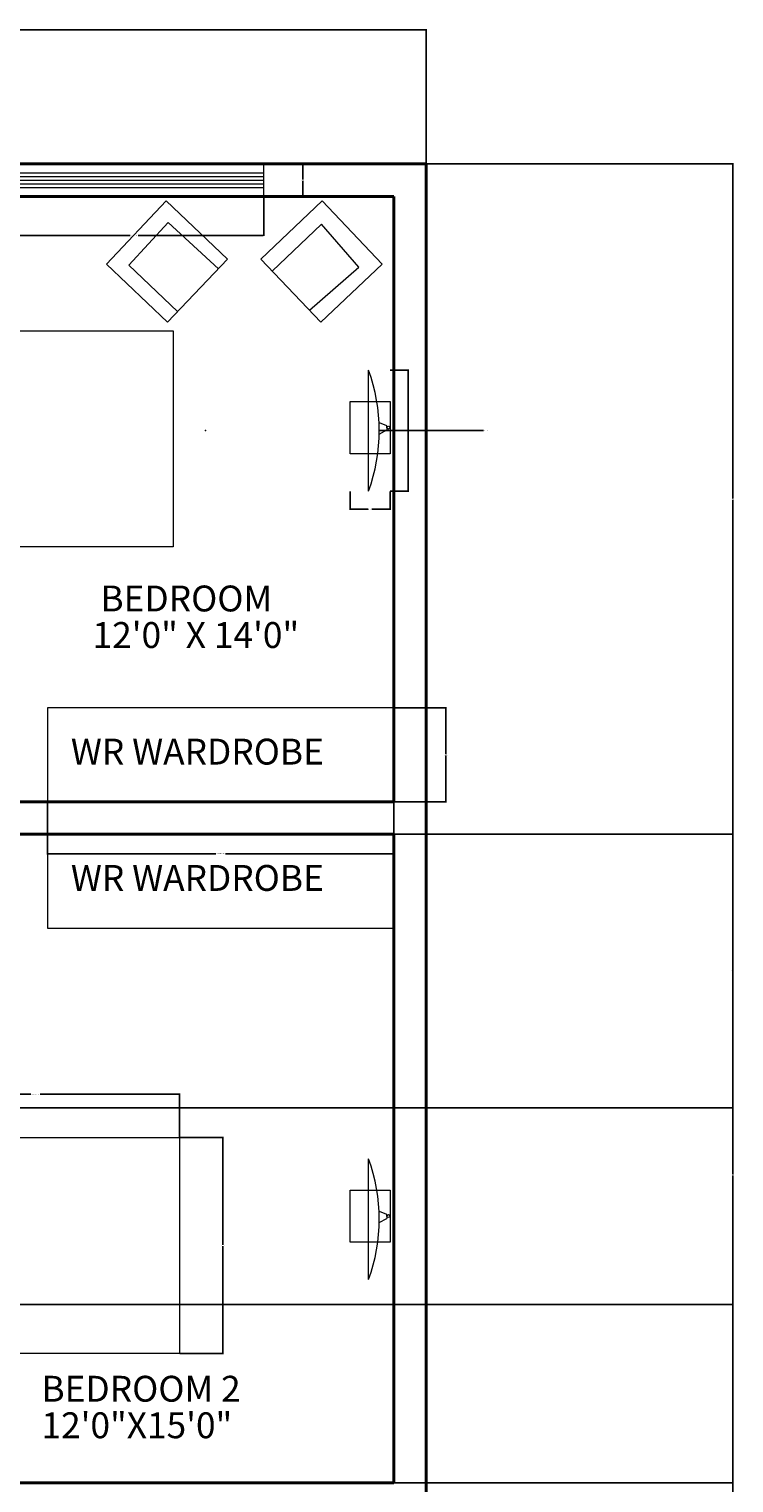
# Model space of a CAD drawing. Units: inches. Extents: x 12978 to 13669, y 46550 to 47327.
# Tile 5 of 5: x 13474 to 13669, y 46901 to 47304. Entities that reach past the tile are written whole.
import ezdxf

# ---------------------------------------------------------------- set-up
doc = ezdxf.new("R2010")
doc.units = ezdxf.units.IN
for name, color, linetype, lineweight in [('A-ANNO-DIMS', 2, 'Continuous', 18), ('A-AREA-IDEN', 1, 'Continuous', 18), ('A-EQPM', 8, 'Continuous', 18), ('A-FLOR-CASE', 8, 'Continuous', 20), ('furniture', 5, 'Continuous', 18), ('text', 1, 'Continuous', 18), ('wall', 7, 'Continuous', 40), ('window', 1, 'Continuous', 18)]:
    doc.layers.add(name, color=color, linetype=linetype, lineweight=lineweight)
doc.styles.get("Standard").update_dxf_attribs({"font": 'arial.ttf'})
doc.dimstyles.get("Standard").update_dxf_attribs({"dimtxt": 0.18, "dimasz": 0.18, "dimexe": 0.18, "dimexo": 0.0625, "dimgap": 0.09, "dimtad": 0, "dimtih": 1, "dimtoh": 1, "dimdec": 4, "dimzin": 0, "dimdsep": 46, "dimtxsty": 'Standard', "dimcen": 0.09, "dimadec": 0, "dimazin": 0, "dimtfac": 1, "dimtdec": 4, "dimtofl": 0, "dimtmove": 0, "dimatfit": 3, "dimfxl": 1, "dimtolj": 1, "dimtzin": 0, "dimarcsym": 0})

# ---------------------------------------------------------------- blocks, each defined once
blk = doc.blocks.new('Bed - Queen')
for p, q in [((0, -80.00003), (0, 0)), ((0, 0), (59.99999, 0)), ((59.99999, 0), (59.99999, -80.00003)), ((7.99999, -1.2), (28.79998, -1.2)), ((7.99999, -14.4), (7.99999, -1.2)), ((28.79998, -1.2), (28.79998, -14.4)), ((31.19999, -1.2), (51.99999, -1.2)), ((31.19999, -14.4), (31.19999, -1.2)), ((51.99999, -1.2), (51.99999, -16.4)), ((0, -14.4), (44.8, -14.4)), ((59.99999, -29.6), (44.8, -14.4)), ((44.8, -14.4), (44.8, -29.6)), ((44.8, -16.8), (0, -16.8)), ((51.99999, -16.4), (46.79936, -16.4)), ((44.8, -29.6), (59.99999, -29.6)), ((59.99999, -80.00003), (0, -80.00003))]:
    blk.add_line(p, q)
blk = doc.blocks.new('WINDOW-72')
for p, q in [((0, 0), (0, 9)), ((72, 0), (72, 9)), ((0, 6.5), (72, 6.5)), ((0, 5.5), (72, 5.5)), ((0, 4.5), (72, 4.5)), ((0, 3.5), (72, 3.5)), ((0, 2.5), (72, 2.5))]:
    blk.add_line(p, q)
blk = doc.blocks.new('TV-FLATSCREEN')
for p, q in [((5.09, 0), (5.09, 33.56)), ((8.05, 19.02), (10.09, 18.18)), ((8.09, 15.82), (10.22, 17.01)), ((10.09, 18.18), (10.22, 17.01)), ((11.07, 17.34), (11.07, 18.07))]:
    blk.add_line(p, q)
blk.add_lwpolyline([(0, 24.86), (11.07, 24.86), (11.07, 10.37), (0, 10.37)], close=True)
blk.add_circle((10.63, 17.63), 0.418)
blk.add_arc((-40.12, 16.78), 48.22, 339.6348, 20.3652)
blk = doc.blocks.new('WARDROBE-96')
blk.add_lwpolyline([(0, 0), (96.12, 0), (96.12, 26.05), (0, 26.05)], close=True)
blk = doc.blocks.new('*D23')
at = {"layer": 'A-ANNO-DIMS', "color": 0, "lineweight": -2, "transparency": 16777216}
for p, q in [((13435.54, 46996.57), (13435.54, 47008.69)), ((13435.72, 47008.51), (13474.24, 47008.51)), ((13515.36, 47008.51), (13476.84, 47008.51)), ((13515.54, 46996.57), (13515.54, 47008.69))]:
    blk.add_line(p, q, dxfattribs=at)
at = {"layer": 'A-ANNO-DIMS', "color": 0, "transparency": 16777216}
for points in [[(13435.72, 47008.54), (13435.72, 47008.48), (13435.54, 47008.51)], [(13515.36, 47008.54), (13515.36, 47008.48), (13515.54, 47008.51)]]:
    blk.add_solid(points, dxfattribs=at)
at = {"layer": 'Defpoints', "color": 0, "transparency": 16777216}
for p in [(13435.54, 47008.51), (13435.54, 46996.51), (13515.54, 46996.51)]:
    blk.add_point(p, dxfattribs=at)
at = {"layer": 'A-ANNO-DIMS', "color": 0, "transparency": 16777216, "insert": (13475.54, 47008.51), "char_height": 0.18, "attachment_point": 5}
blk.add_mtext('\\A1;QUEEN BED 80 TYP.', dxfattribs=at)
blk = doc.blocks.new('*D24')
at = {"layer": 'A-ANNO-DIMS', "color": 0, "lineweight": -2, "transparency": 16777216}
for p, q in [((13515.6, 46996.51), (13527.72, 46996.51)), ((13527.54, 46996.33), (13527.54, 46966.69)), ((13527.54, 46936.69), (13527.54, 46966.33)), ((13515.6, 46936.51), (13527.72, 46936.51))]:
    blk.add_line(p, q, dxfattribs=at)
at = {"layer": 'A-ANNO-DIMS', "color": 0, "transparency": 16777216}
for points in [[(13527.51, 46996.33), (13527.57, 46996.33), (13527.54, 46996.51)], [(13527.51, 46936.69), (13527.57, 46936.69), (13527.54, 46936.51)]]:
    blk.add_solid(points, dxfattribs=at)
at = {"layer": 'Defpoints', "color": 0, "transparency": 16777216}
for p in [(13515.54, 46996.51), (13527.54, 46996.51), (13515.54, 46936.51)]:
    blk.add_point(p, dxfattribs=at)
at = {"layer": 'A-ANNO-DIMS', "color": 0, "transparency": 16777216, "insert": (13527.54, 46966.51), "char_height": 0.18, "attachment_point": 5}
blk.add_mtext('\\A1;60 TYP.', dxfattribs=at)
blk = doc.blocks.new('*D29')
at = {"layer": 'A-ANNO-DIMS', "color": 0, "lineweight": -2, "transparency": 16777216}
for p, q in [((13574.01, 47209.41), (13579.16, 47209.41)), ((13578.98, 47209.23), (13578.98, 47192.82)), ((13578.98, 47176.03), (13578.98, 47192.45)), ((13574.01, 47175.85), (13579.16, 47175.85))]:
    blk.add_line(p, q, dxfattribs=at)
at = {"layer": 'A-ANNO-DIMS', "color": 0, "transparency": 16777216}
for points in [[(13578.95, 47209.23), (13579.01, 47209.23), (13578.98, 47209.41)], [(13578.95, 47176.03), (13579.01, 47176.03), (13578.98, 47175.85)]]:
    blk.add_solid(points, dxfattribs=at)
at = {"layer": 'Defpoints', "color": 0, "transparency": 16777216}
for p in [(13573.95, 47209.41), (13578.98, 47209.41), (13573.95, 47175.85)]:
    blk.add_point(p, dxfattribs=at)
at = {"layer": 'A-ANNO-DIMS', "color": 0, "transparency": 16777216, "insert": (13578.98, 47192.63), "char_height": 0.18, "attachment_point": 5}
blk.add_mtext('\\A1;TV 34 TYP.', dxfattribs=at)
blk = doc.blocks.new('*D30')
at = {"layer": 'A-ANNO-DIMS', "color": 0, "lineweight": -2, "transparency": 16777216}
for p, q in [((13562.88, 47175.79), (13562.88, 47170.64)), ((13573.95, 47175.79), (13573.95, 47170.64)), ((13563.06, 47170.82), (13567.89, 47170.82)), ((13573.77, 47170.82), (13568.93, 47170.82))]:
    blk.add_line(p, q, dxfattribs=at)
at = {"layer": 'A-ANNO-DIMS', "color": 0, "transparency": 16777216}
for points in [[(13563.06, 47170.85), (13563.06, 47170.79), (13562.88, 47170.82)], [(13573.77, 47170.85), (13573.77, 47170.79), (13573.95, 47170.82)]]:
    blk.add_solid(points, dxfattribs=at)
at = {"layer": 'Defpoints', "color": 0, "transparency": 16777216}
for p in [(13562.88, 47175.85), (13573.95, 47175.85), (13573.95, 47170.82)]:
    blk.add_point(p, dxfattribs=at)
at = {"layer": 'A-ANNO-DIMS', "color": 0, "transparency": 16777216, "insert": (13568.41, 47170.82), "char_height": 0.18, "attachment_point": 5}
blk.add_mtext('\\A1;11 TYP.', dxfattribs=at)
blk = doc.blocks.new('*D31')
at = {"layer": 'A-ANNO-DIMS', "color": 0, "lineweight": -2, "transparency": 16777216}
for p, q in [((13478.89, 47089.57), (13478.89, 47075.04)), ((13575.01, 47089.57), (13575.01, 47075.04)), ((13479.07, 47075.22), (13525.64, 47075.22)), ((13574.83, 47075.22), (13528.25, 47075.22))]:
    blk.add_line(p, q, dxfattribs=at)
at = {"layer": 'A-ANNO-DIMS', "color": 0, "transparency": 16777216}
for points in [[(13479.07, 47075.25), (13479.07, 47075.19), (13478.89, 47075.22)], [(13574.83, 47075.25), (13574.83, 47075.19), (13575.01, 47075.22)]]:
    blk.add_solid(points, dxfattribs=at)
at = {"layer": 'Defpoints', "color": 0, "transparency": 16777216}
for p in [(13478.89, 47089.63), (13575.01, 47089.63), (13575.01, 47075.22)]:
    blk.add_point(p, dxfattribs=at)
at = {"layer": 'A-ANNO-DIMS', "color": 0, "transparency": 16777216, "insert": (13526.95, 47075.22), "char_height": 0.18, "attachment_point": 5}
blk.add_mtext('\\A1;WARDROBE 96 TYP.', dxfattribs=at)
blk = doc.blocks.new('*D32')
at = {"layer": 'A-ANNO-DIMS', "color": 0, "lineweight": -2, "transparency": 16777216}
for p, q in [((13575.07, 47115.69), (13589.6, 47115.69)), ((13589.42, 47115.51), (13589.42, 47102.84)), ((13589.42, 47089.81), (13589.42, 47102.48)), ((13575.07, 47089.63), (13589.6, 47089.63))]:
    blk.add_line(p, q, dxfattribs=at)
at = {"layer": 'A-ANNO-DIMS', "color": 0, "transparency": 16777216}
for points in [[(13589.39, 47115.51), (13589.45, 47115.51), (13589.42, 47115.69)], [(13589.39, 47089.81), (13589.45, 47089.81), (13589.42, 47089.63)]]:
    blk.add_solid(points, dxfattribs=at)
at = {"layer": 'Defpoints', "color": 0, "transparency": 16777216}
for p in [(13575.01, 47115.69), (13589.42, 47115.69), (13575.01, 47089.63)]:
    blk.add_point(p, dxfattribs=at)
at = {"layer": 'A-ANNO-DIMS', "color": 0, "transparency": 16777216, "insert": (13589.42, 47102.66), "char_height": 0.18, "attachment_point": 5}
blk.add_mtext('\\A1;26 TYP.', dxfattribs=at)
blk = doc.blocks.new('*D33')
at = {"layer": 'A-ANNO-DIMS', "color": 0, "lineweight": -2, "transparency": 16777216}
for p, q in [((13466.96, 47257.57), (13466.96, 47246.65)), ((13538.96, 47257.57), (13538.96, 47246.65)), ((13467.14, 47246.83), (13501.84, 47246.83)), ((13538.78, 47246.83), (13504.08, 47246.83))]:
    blk.add_line(p, q, dxfattribs=at)
at = {"layer": 'A-ANNO-DIMS', "color": 0, "transparency": 16777216}
for points in [[(13467.14, 47246.86), (13467.14, 47246.8), (13466.96, 47246.83)], [(13538.78, 47246.86), (13538.78, 47246.8), (13538.96, 47246.83)]]:
    blk.add_solid(points, dxfattribs=at)
at = {"layer": 'Defpoints', "color": 0, "transparency": 16777216}
for p in [(13466.96, 47257.63), (13538.96, 47257.63), (13538.96, 47246.83)]:
    blk.add_point(p, dxfattribs=at)
at = {"layer": 'A-ANNO-DIMS', "color": 0, "transparency": 16777216, "insert": (13502.96, 47246.83), "char_height": 0.18, "attachment_point": 5}
blk.add_mtext('\\A1;WINDOW 72 TYP.', dxfattribs=at)
blk = doc.blocks.new('*D34')
at = {"layer": 'A-ANNO-DIMS', "color": 0, "lineweight": -2, "transparency": 16777216}
for p, q in [((13539.02, 47266.63), (13549.94, 47266.63)), ((13549.76, 47266.45), (13549.76, 47262.32)), ((13549.76, 47257.81), (13549.76, 47261.95)), ((13539.02, 47257.63), (13549.94, 47257.63))]:
    blk.add_line(p, q, dxfattribs=at)
at = {"layer": 'A-ANNO-DIMS', "color": 0, "transparency": 16777216}
for points in [[(13549.73, 47266.45), (13549.79, 47266.45), (13549.76, 47266.63)], [(13549.73, 47257.81), (13549.79, 47257.81), (13549.76, 47257.63)]]:
    blk.add_solid(points, dxfattribs=at)
at = {"layer": 'Defpoints', "color": 0, "transparency": 16777216}
for p in [(13538.96, 47266.63), (13549.76, 47266.63), (13538.96, 47257.63)]:
    blk.add_point(p, dxfattribs=at)
at = {"layer": 'A-ANNO-DIMS', "color": 0, "transparency": 16777216, "insert": (13549.76, 47262.13), "char_height": 0.18, "attachment_point": 5}
blk.add_mtext('\\A1;9 TYP.', dxfattribs=at)
blk = doc.blocks.new('*D51')
at = {"layer": 'A-ANNO-DIMS', "color": 0, "lineweight": -2, "transparency": 16777216}
for p, q in [((13059.01, 47266.7), (13059.01, 47304.06)), ((13059.19, 47303.88), (13321.22, 47303.88)), ((13583.83, 47303.88), (13321.79, 47303.88)), ((13584.01, 47266.7), (13584.01, 47304.06))]:
    blk.add_line(p, q, dxfattribs=at)
at = {"layer": 'A-ANNO-DIMS', "color": 0, "transparency": 16777216}
for points in [[(13059.19, 47303.91), (13059.19, 47303.85), (13059.01, 47303.88)], [(13583.83, 47303.91), (13583.83, 47303.85), (13584.01, 47303.88)]]:
    blk.add_solid(points, dxfattribs=at)
at = {"layer": 'Defpoints', "color": 0, "transparency": 16777216}
for p in [(13584.01, 47303.88), (13059.01, 47266.63), (13584.01, 47266.63)]:
    blk.add_point(p, dxfattribs=at)
at = {"layer": 'A-ANNO-DIMS', "color": 0, "transparency": 16777216, "insert": (13321.51, 47303.88), "char_height": 0.18, "attachment_point": 5}
blk.add_mtext('\\A1;525', dxfattribs=at)
blk = doc.blocks.new('*D57')
at = {"layer": 'A-ANNO-DIMS', "color": 0, "lineweight": -2, "transparency": 16777216}
for p, q in [((13575.07, 47080.63), (13669.26, 47080.63)), ((13669.08, 47080.45), (13669.08, 46986.32)), ((13669.08, 46891.81), (13669.08, 46985.95)), ((13584.07, 46891.63), (13669.26, 46891.63))]:
    blk.add_line(p, q, dxfattribs=at)
at = {"layer": 'A-ANNO-DIMS', "color": 0, "transparency": 16777216}
for points in [[(13669.05, 47080.45), (13669.11, 47080.45), (13669.08, 47080.63)], [(13669.05, 46891.81), (13669.11, 46891.81), (13669.08, 46891.63)]]:
    blk.add_solid(points, dxfattribs=at)
at = {"layer": 'Defpoints', "color": 0, "transparency": 16777216}
for p in [(13575.01, 47080.63), (13669.08, 47080.63), (13584.01, 46891.63)]:
    blk.add_point(p, dxfattribs=at)
at = {"layer": 'A-ANNO-DIMS', "color": 0, "transparency": 16777216, "insert": (13669.08, 46986.13), "char_height": 0.18, "attachment_point": 5}
blk.add_mtext('\\A1;189', dxfattribs=at)
blk = doc.blocks.new('*D58')
at = {"layer": 'A-ANNO-DIMS', "color": 0, "lineweight": -2, "transparency": 16777216}
for p, q in [((13584.07, 47266.63), (13669.26, 47266.63)), ((13669.08, 47266.45), (13669.08, 47173.82)), ((13669.08, 47080.81), (13669.08, 47173.45)), ((13575.07, 47080.63), (13669.26, 47080.63))]:
    blk.add_line(p, q, dxfattribs=at)
at = {"layer": 'A-ANNO-DIMS', "color": 0, "transparency": 16777216}
for points in [[(13669.05, 47266.45), (13669.11, 47266.45), (13669.08, 47266.63)], [(13669.05, 47080.81), (13669.11, 47080.81), (13669.08, 47080.63)]]:
    blk.add_solid(points, dxfattribs=at)
at = {"layer": 'Defpoints', "color": 0, "transparency": 16777216}
for p in [(13584.01, 47266.63), (13669.08, 47266.63), (13575.01, 47080.63)]:
    blk.add_point(p, dxfattribs=at)
at = {"layer": 'A-ANNO-DIMS', "color": 0, "transparency": 16777216, "insert": (13669.08, 47173.63), "char_height": 0.18, "attachment_point": 5}
blk.add_mtext('\\A1;186', dxfattribs=at)
blk = doc.blocks.new('*D72')
at = {"layer": 'A-ANNO-DIMS', "color": 0, "lineweight": -2, "transparency": 16777216}
for p, q in [((13188.07, 46950.13), (13669.26, 46950.13)), ((13669.08, 46949.95), (13669.08, 46925.57)), ((13669.08, 46900.81), (13669.08, 46925.2)), ((13188.07, 46900.63), (13669.26, 46900.63))]:
    blk.add_line(p, q, dxfattribs=at)
at = {"layer": 'A-ANNO-DIMS', "color": 0, "transparency": 16777216}
for points in [[(13669.05, 46949.95), (13669.11, 46949.95), (13669.08, 46950.13)], [(13669.05, 46900.81), (13669.11, 46900.81), (13669.08, 46900.63)]]:
    blk.add_solid(points, dxfattribs=at)
at = {"layer": 'Defpoints', "color": 0, "transparency": 16777216}
for p in [(13188.01, 46950.13), (13669.08, 46950.13), (13188.01, 46900.63)]:
    blk.add_point(p, dxfattribs=at)
at = {"layer": 'A-ANNO-DIMS', "color": 0, "transparency": 16777216, "insert": (13669.08, 46925.38), "char_height": 0.18, "attachment_point": 5}
blk.add_mtext('\\A1;49.5', dxfattribs=at)
blk = doc.blocks.new('*D73')
at = {"layer": 'A-ANNO-DIMS', "color": 0, "lineweight": -2, "transparency": 16777216}
for p, q in [((13200.07, 47080.63), (13669.26, 47080.63)), ((13669.08, 47080.45), (13669.08, 47042.85)), ((13669.08, 47004.87), (13669.08, 47042.48)), ((13200.07, 47004.69), (13669.26, 47004.69))]:
    blk.add_line(p, q, dxfattribs=at)
at = {"layer": 'A-ANNO-DIMS', "color": 0, "transparency": 16777216}
for points in [[(13669.05, 47080.45), (13669.11, 47080.45), (13669.08, 47080.63)], [(13669.05, 47004.87), (13669.11, 47004.87), (13669.08, 47004.69)]]:
    blk.add_solid(points, dxfattribs=at)
at = {"layer": 'Defpoints', "color": 0, "transparency": 16777216}
for p in [(13200.01, 47080.63), (13669.08, 47080.63), (13200.01, 47004.69)]:
    blk.add_point(p, dxfattribs=at)
at = {"layer": 'A-ANNO-DIMS', "color": 0, "transparency": 16777216, "insert": (13669.08, 47042.66), "char_height": 0.18, "attachment_point": 5}
blk.add_mtext('\\A1;75.94', dxfattribs=at)
blk = doc.blocks.new('*D81')
at = {"layer": 'A-ANNO-DIMS', "color": 0, "lineweight": -2, "transparency": 16777216}
for p, q in [((13522.67, 47192.63), (13522.85, 47192.63)), ((13522.76, 47192.54), (13522.76, 47192.72)), ((13599.91, 47192.63), (13571.16, 47192.63))]:
    blk.add_line(p, q, dxfattribs=at)
at = {"layer": 'A-ANNO-DIMS', "color": 0, "transparency": 16777216}
blk.add_solid([(13571.16, 47192.66), (13571.16, 47192.6), (13570.98, 47192.63)], dxfattribs=at)
at = {"layer": 'Defpoints', "color": 0, "transparency": 16777216}
for p in [(13522.76, 47192.63), (13570.98, 47192.63)]:
    blk.add_point(p, dxfattribs=at)
at = {"layer": 'A-ANNO-DIMS', "color": 0, "transparency": 16777216, "insert": (13600.58, 47192.63), "char_height": 0.18, "attachment_point": 5}
blk.add_mtext('\\A1;3X R48.22', dxfattribs=at)

msp = doc.modelspace()

# ---------------------------------------------------------------- linework, layer by layer
at = {"layer": 'furniture'}
for p, q in [((13512.3335, 47250.401), (13501.4323, 47238.5265)), ((13526.3127, 47237.5676), (13512.3335, 47250.401)), ((13554.961, 47249.9047), (13541.2656, 47236.902)), ((13565.3192, 47238.0366), (13554.961, 47249.9047)), ((13501.4323, 47238.5265), (13514.9964, 47225.6484)), ((13551.5762, 47226.0421), (13565.3192, 47238.0366))]:
    msp.add_line(p, q, dxfattribs=at)
for points in [[(13495.2194, 47238.8609), (13511.8576, 47256.3855), (13528.8562, 47240.2466), (13512.2181, 47222.722)], [(13571.727, 47238.8609), (13555.0889, 47256.3855), (13538.0902, 47240.2466), (13554.7284, 47222.722)]]:
    msp.add_lwpolyline(points, close=True, dxfattribs=at)
at = {"layer": 'wall'}
for p, q in [((13059.005, 47266.6345), (13584.005, 47266.6345)), ((13584.005, 47266.6345), (13584.005, 46891.6345)), ((13431.005, 47257.6345), (13575.005, 47257.6345)), ((13575.005, 47257.6345), (13575.005, 47089.6345)), ((13431.005, 47089.6345), (13575.005, 47089.6345)), ((13431.005, 47080.6345), (13575.005, 47080.6345)), ((13575.005, 47080.6345), (13575.005, 46900.6345)), ((13431.005, 46900.6345), (13575.005, 46900.6345))]:
    msp.add_line(p, q, dxfattribs=at)

# ---------------------------------------------------------------- block references
at = {"layer": 'A-EQPM'}
for p in [(13562.8773, 47175.8548), (13562.8773, 46957.043)]:
    msp.add_blockref('TV-FLATSCREEN', p, dxfattribs=at)
at = {"layer": 'A-FLOR-CASE'}
for p in [(13478.8851, 47089.6345), (13478.8851, 47054.5813)]:
    msp.add_blockref('WARDROBE-96', p, dxfattribs=at)
at = {"layer": 'furniture', "rotation": 90}
for p in [(13433.7494, 47160.3603), (13435.5385, 46936.511)]:
    msp.add_blockref('Bed - Queen', p, dxfattribs=at)
at = {"layer": 'window'}
msp.add_blockref('WINDOW-72', (13466.959, 47257.6345), dxfattribs=at)

# ---------------------------------------------------------------- texts
at = {"layer": 'A-AREA-IDEN'}
for s, height, p in [(' BEDROOM', 7.17855, (13491.393, 47142.4672)), ('12\'0" X 14\'0"', 7.178549, (13491.393, 47132.3288)), ('BEDROOM 2', 7.17855, (13477.2159, 46923.1774)), ('12\'0"X15\'0"', 7.178549, (13477.2159, 46913.0389))]:
    msp.add_text(s, height=height, dxfattribs=at).set_placement(p)
at = {"layer": 'text'}
for p in [(13485.3737, 47099.97), (13485.3737, 47064.9168)]:
    msp.add_text('WR WARDROBE', height=7.178549, dxfattribs=at).set_placement(p)

# ---------------------------------------------------------------- dimensions: what is measured, and where the dimension line sits
at = {"layer": 'A-ANNO-DIMS'}
dim = msp.add_linear_dim(base=(13584.005, 47303.8845), p1=(13059.005, 47266.6345), p2=(13584.005, 47266.6345), dimstyle='Standard', override={"dimdec": 0, "dimlfac": 1, "dimrnd": 0, "dimzin": 0, "dimdsep": 46, "dimlunit": 2}, dxfattribs=at)
dim.commit()
dim.dimension.update_dxf_attribs({"geometry": '*D51', "text_midpoint": (13321.505, 47303.8845)})
for base, p1, p2, angle, text, picture, middle in [((13549.759, 47266.6345), (13538.959, 47257.6345), (13538.959, 47266.6345), 90, '<> TYP.', '*D34', (13549.759, 47262.1345)), ((13578.9822, 47209.4132), (13573.9485, 47175.8548), (13573.9485, 47209.4132), 90, 'TV <> TYP.', '*D29', (13578.9822, 47192.634)), ((13589.423, 47115.6876), (13575.005, 47089.6345), (13575.005, 47115.6876), 90, '<> TYP.', '*D32', (13589.423, 47102.661)), ((13435.5385, 47008.511), (13515.5385, 46996.511), (13435.5385, 46996.511), 180, 'QUEEN BED <> TYP.', '*D23', (13475.5385, 47008.511)), ((13527.5385, 46996.511), (13515.5385, 46936.511), (13515.5385, 46996.511), 90, '<> TYP.', '*D24', (13527.5385, 46966.511))]:
    dim = msp.add_linear_dim(base=base, p1=p1, p2=p2, angle=angle, text=text, dimstyle='Standard', override={"dimdec": 0, "dimlfac": 1, "dimrnd": 0, "dimzin": 0, "dimdsep": 46, "dimlunit": 2}, dxfattribs=at)
    dim.commit()
    dim.dimension.update_dxf_attribs({"geometry": picture, "text_midpoint": middle})
for base, p1, p2, override, picture, middle in [((13669.0793, 47266.6345), (13575.005, 47080.6345), (13584.005, 47266.6345), {"dimdec": 0, "dimlfac": 1, "dimrnd": 0, "dimzin": 0, "dimdsep": 46, "dimlunit": 2}, '*D58', (13669.0793, 47173.6345)), ((13669.0793, 47080.6345), (13200.005, 47004.6918), (13200.005, 47080.6345), {"dimdec": 2, "dimlfac": 1, "dimrnd": 0, "dimzin": 0, "dimdsep": 46, "dimlunit": 2}, '*D73', (13669.0793, 47042.6631)), ((13669.0793, 47080.6345), (13584.005, 46891.6345), (13575.005, 47080.6345), {"dimdec": 0, "dimlfac": 1, "dimrnd": 0, "dimzin": 0, "dimdsep": 46, "dimlunit": 2}, '*D57', (13669.0793, 46986.1345)), ((13669.0793, 46950.1345), (13188.005, 46900.6345), (13188.005, 46950.1345), {"dimdec": 1, "dimlfac": 1, "dimrnd": 0, "dimzin": 0, "dimdsep": 46, "dimlunit": 2}, '*D72', (13669.0793, 46925.3845))]:
    dim = msp.add_linear_dim(base=base, p1=p1, p2=p2, angle=90, dimstyle='Standard', override=override, dxfattribs=at)
    dim.commit()
    dim.dimension.update_dxf_attribs({"geometry": picture, "text_midpoint": middle})
for base, p1, p2, text, picture, middle in [((13538.959, 47246.8345), (13466.959, 47257.6345), (13538.959, 47257.6345), 'WINDOW <> TYP.', '*D33', (13502.959, 47246.8345)), ((13573.9485, 47170.8211), (13562.8773, 47175.8548), (13573.9485, 47175.8548), '<> TYP.', '*D30', (13568.4129, 47170.8211)), ((13575.005, 47075.2165), (13478.8851, 47089.6345), (13575.005, 47089.6345), 'WARDROBE <> TYP.', '*D31', (13526.9451, 47075.2165))]:
    dim = msp.add_linear_dim(base=base, p1=p1, p2=p2, text=text, dimstyle='Standard', override={"dimdec": 0, "dimlfac": 1, "dimrnd": 0, "dimzin": 0, "dimdsep": 46, "dimlunit": 2}, dxfattribs=at)
    dim.commit()
    dim.dimension.update_dxf_attribs({"geometry": picture, "text_midpoint": middle})
dim = msp.add_radius_dim(center=(13522.7615, 47192.634), mpoint=(13570.9772, 47192.634), text='3X <>', dimstyle='Standard', override={"dimdec": 2, "dimlfac": 1, "dimrnd": 0, "dimzin": 0, "dimdsep": 46, "dimlunit": 2}, dxfattribs=at)
dim.commit()
dim.dimension.update_dxf_attribs({"geometry": '*D81', "text_midpoint": (13599.9066, 47192.634), "dimtype": 164})

doc.saveas('drawing.dxf')
